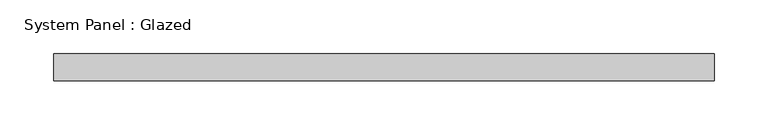
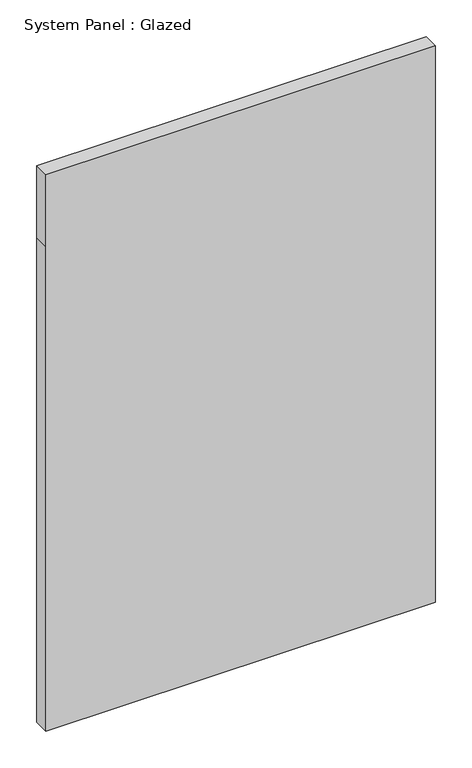
"""IFC4 building model written with IfcOpenShell, lengths in millimetres: plate geometry, System Panel : Glazed."""

from ifc_helpers import new_model, si_unit, frame, origin, place, context, project, spatial, polyline, outline, extrude, source, transform, mapped, element, save


def system_panel_glazed_c7c048a3(model_context):
    return source(origin(), model_context, "Body", "SweptSolid", [
        extrude(outline(polyline([(0.0, -307.975), (0.0, 307.975), (810.0902035, 307.975), (930.7402035, 307.975), (930.7402035, -307.975), (810.0902035, -307.975), (0.0, -307.975)])), frame((0.0, 19.05, 0.0), z_axis=(0.0, 1.0, 0.0), x_axis=(0.0, 0.0, 1.0)), (0.0, 0.0, 1.0), 25.4),
    ])


if __name__ == "__main__":
    model = new_model("IFC4")
    model_context = context("Model", 3, world=origin())
    ifc_project = project(units=[si_unit("LENGTHUNIT", "METRE", prefix="MILLI")], contexts=[model_context])
    site = spatial("IfcSite", under=ifc_project)
    building = spatial("IfcBuilding", under=site)
    placement = place(None, origin())
    system_panel_glazed_shape = system_panel_glazed_c7c048a3(model_context)
    element("IfcPlate", 1, ObjectType="System Panel : Glazed", at=placement, inside=building, context=model_context, shape_type="MappedRepresentation", body=[
        mapped(system_panel_glazed_shape, transform((0.0, 0.0, 0.0), x_axis=(1.0, 0.0, 0.0), y_axis=(0.0, 1.0, 0.0), z_axis=(0.0, 0.0, 1.0))),
    ])
    save(model, "model.ifc")

# Revit data of these elements
# Type "System Panel : Glazed"
#   Construction Type Id = "GSP4R"
#   Analytic Construction = "1/8 in Pilkington single glazing"
#   Visual Light Transmittance = 0.9
#   Solar Heat Gain Coefficient = 0.86
#   Heat Transfer Coefficient (U) = 1.18115 BTU/(h·ft²·°F)
#   Define Thermal Properties by = 1
# Element 1 (IfcPlate, "System Panel : Glazed")
#   Materials on its faces: "Glass"
# Materials
#   "Glass": class "Glass", colour RGB 0 128 192, transparency 0.75, Description = "Soda Lime Glass", Cost = 0
